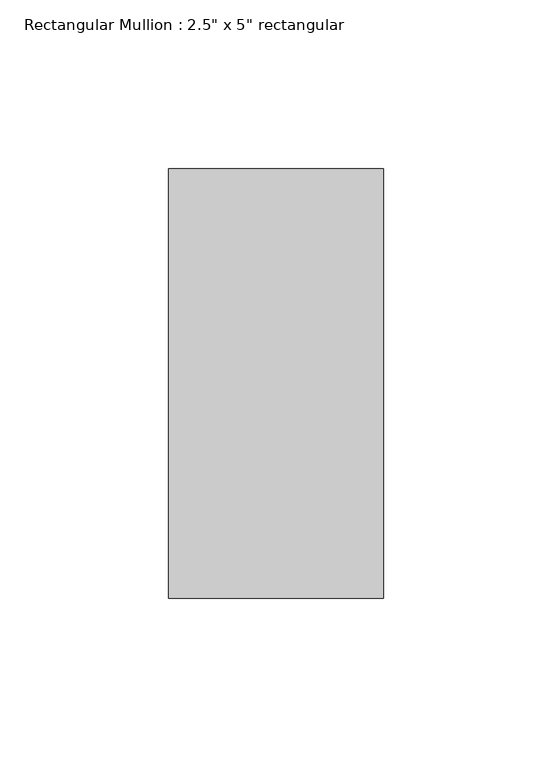
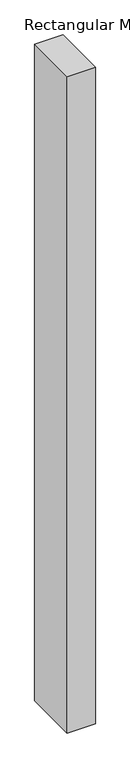
"""IFC4 building model written with IfcOpenShell, lengths in millimetres: member geometry."""

from ifc_helpers import new_model, si_unit, frame, origin, place, context, project, spatial, polyline, outline, extrude, source, transform, mapped, element, save


def member_104ec00a(model_context):
    return source(origin(), model_context, "Body", "SweptSolid", [
        extrude(outline(polyline([(31.75, 63.5), (31.75, -63.5), (-31.75, -63.5), (-31.75, 63.5), (31.75, 63.5)])), frame((0.0, 0.0, -1566.7320436), z_axis=(0.0, 0.0, 1.0), x_axis=(1.0, 0.0, 0.0)), (0.0, 0.0, 1.0), 1566.7320436),
    ])


if __name__ == "__main__":
    model = new_model("IFC4")
    model_context = context("Model", 3, world=origin())
    ifc_project = project(units=[si_unit("LENGTHUNIT", "METRE", prefix="MILLI")], contexts=[model_context])
    site = spatial("IfcSite", under=ifc_project)
    building = spatial("IfcBuilding", under=site)
    placement = place(None, origin())
    member_shape = member_104ec00a(model_context)
    element("IfcMember", 1, ObjectType="Rectangular Mullion : 2.5\" x 5\" rectangular", at=placement, inside=building, context=model_context, shape_type="MappedRepresentation", body=[
        mapped(member_shape, transform((0.0, 0.0, 0.0), x_axis=(1.0, 0.0, 0.0), y_axis=(0.0, 1.0, 0.0), z_axis=(0.0, 0.0, 1.0))),
    ])
    save(model, "model.ifc")

# Revit data of these elements
# Type "Rectangular Mullion : 2.5\" x 5\" rectangular"
#   built-in parameter 1007304 = 0.416667 (stored number, unit not read)
#   built-in parameter 1007301 = 0.104167 (stored number, unit not read)
#   built-in parameter 1007300 = 0.104167 (stored number, unit not read)
# Element 1 (IfcMember, "Rectangular Mullion : 2.5\" x 5\" rectangular")
#   Materials on its faces: "Aluminum"
# Materials
#   "Aluminum": class "Metal", colour RGB 247 247 247, transparency 0, Description = "Aluminum 6061", Cost = 0
